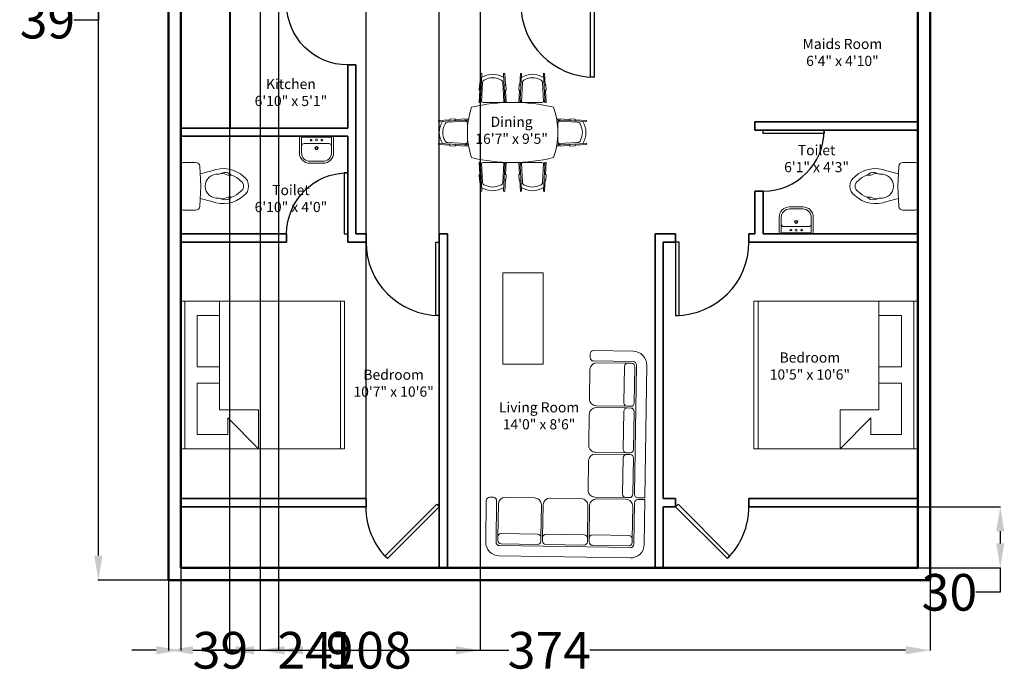
# Model space of a CAD drawing. Units: inches. Extents: x -230 to 384, y -962 to -183.
# Tile 1 of 6: x -175 to 309, y -962 to -640. Entities that reach past the tile are written whole.
import ezdxf

# ---------------------------------------------------------------- set-up
doc = ezdxf.new("R2010")
doc.units = ezdxf.units.IN
for name, color, linetype, lineweight in [('A-ANNO-DIMS', 2, 'Continuous', 18), ('A-AREA-IDEN', 7, 'Continuous', 18), ('A-DOOR', 3, 'Continuous', 25), ('A-FLOR-FIXT', 9, 'Continuous', 18), ('Furniture', 2, 'Continuous', 18), ('Inner Wall', 5, 'Continuous', 35), ('Kitchen', 4, 'Continuous', 25), ('Outer Wall', 1, 'Continuous', 50)]:
    doc.layers.add(name, color=color, linetype=linetype, lineweight=lineweight)
doc.styles.get("Standard").update_dxf_attribs({"font": 'arial.ttf'})
doc.dimstyles.get("Standard").update_dxf_attribs({"dimtxt": 18, "dimasz": 12, "dimexe": 0.18, "dimexo": 0.0625, "dimgap": 0.09, "dimtad": 0, "dimtih": 1, "dimtoh": 1, "dimdec": 0, "dimzin": 0, "dimdsep": 46, "dimlunit": 3, "dimtxsty": 'Standard', "dimcen": 0.09, "dimadec": 0, "dimazin": 0, "dimtfac": 1, "dimtdec": 0, "dimtofl": 0, "dimtmove": 0, "dimatfit": 3, "dimfxl": 1, "dimtolj": 1, "dimtzin": 0, "dimarcsym": 0})

# ---------------------------------------------------------------- blocks, each defined once
blk = doc.blocks.new('*U4')
for p, q in [((0, 0), (0, -4)), ((36, 0), (36, -4))]:
    blk.add_line(p, q)
blk.add_lwpolyline([(0, 0), (0, 36), (1.75, 36), (1.75, 0)], close=True)
blk.add_arc((0, 0), 36, 0, 90)
blk = doc.blocks.new('*U2')
for p, q in [((0, 0), (0, 4)), ((36, 0), (36, 4))]:
    blk.add_line(p, q)
blk.add_lwpolyline([(0, 0), (0, -36), (1.75, -36), (1.75, 0)], close=True)
blk.add_arc((0, 0), 36, 270, 0)
blk = doc.blocks.new('*U5')
for p, q in [((0, 0), (0, 4)), ((36, 0), (36, 4))]:
    blk.add_line(p, q)
blk.add_lwpolyline([(0, 0), (25.46, -25.46), (26.69, -24.22), (1.24, 1.24)], close=True)
blk.add_arc((0, 0), 36, 315, 0)
blk = doc.blocks.new('*U6')
for p, q in [((0, 0), (0, -4)), ((30, 0), (30, -4))]:
    blk.add_line(p, q)
blk.add_lwpolyline([(0, 0), (0, 30), (1.75, 30), (1.75, 0)], close=True)
blk.add_arc((0, 0), 30, 0, 90)
blk = doc.blocks.new('KING-00')
for p, q in [((-0.897, -0.947), (-0.897, 0.882)), ((0.602, 0.882), (0.602, -0.464)), ((1.034, -0.947), (1.034, 0.882)), ((0.602, 0.704), (0.881, 0.704)), ((0.881, 0.069), (0.881, 0.704)), ((0.602, 0.069), (0.881, 0.069)), ((0.881, -0.134), (0.602, -0.134)), ((0.881, -0.769), (0.881, -0.134)), ((0.119, -0.464), (0.119, -0.947)), ((0.602, -0.464), (0.119, -0.464)), ((0.119, -0.947), (0.5, -0.566)), ((0.5, -0.769), (0.5, -0.566)), ((0.5, -0.769), (0.881, -0.769))]:
    blk.add_line(p, q)
blk.add_lwpolyline([(-0.948, -0.947), (-0.948, 0.882), (1.084, 0.882), (1.084, -0.947)], close=True)
blk = doc.blocks.new('A$C1308471B')
at = {"ltscale": 20}
for p, q in [((0, 0.4607), (0, 0.0186)), ((0.0354, 0.4793), (0.1495, 0.4793)), ((0.2013, 0.2397), (0.1923, 0.4384)), ((0.1957, 0.3639), (0.3109, 0.3953)), ((0.5021, 0.3528), (0.4724, 0.3528)), ((0.4982, 0.3575), (0.4822, 0.3709)), ((0.2013, 0.2397), (0.1923, 0.0409)), ((0.1959, 0.1193), (0.3109, 0.0879)), ((0.5021, 0.1304), (0.4724, 0.1304)), ((0.4982, 0.1257), (0.4822, 0.1123)), ((0.0354, 0), (0.1495, 0))]:
    blk.add_line(p, q, dxfattribs=at)
for centre, radius, start, end in [((0.006, 0.4607), 0.006, 136.52689, 180), ((0.0354, 0.4328), 0.0465, 90, 136.52689), ((0.1495, 0.4365), 0.0429, 2.57554, 90), ((0.4248, 0.1104), 0.3068, 47.41345, 111.79241), ((0.3654, 0.2416), 0.1206, 83.35226, 180), ((0.3823, 0.3868), 0.0255, 263.35226, 298.57415), ((0.4494, 0.2636), 0.1148, 79.39683, 118.57415), ((0.405, 0.2159), 0.153, 63.50202, 90.45216), ((0.4658, 0.3513), 0.0255, 50, 79.39683), ((0.5146, 0.377), 0.0255, 230, 251.38812), ((0.5021, 0.3273), 0.0255, 70.3751, 90), ((0.4248, 0.1104), 0.2558, 46.61198, 70.3751), ((0.5654, 0.2416), 0.116, 0, 54.71147), ((0.3654, 0.2416), 0.1206, 180, 276.64774), ((0.5654, 0.2416), 0.065, 0, 57.29738), ((0.5654, 0.2416), 0.065, 302.70262, 0), ((0.5654, 0.2416), 0.116, 305.28853, 0), ((0.4248, 0.3728), 0.3068, 248.20759, 312.58655), ((0.3823, 0.0964), 0.0255, 61.42585, 96.64774), ((0.4494, 0.2196), 0.1148, 241.42585, 280.60317), ((0.405, 0.2673), 0.153, 269.54784, 296.49798), ((0.4658, 0.1319), 0.0255, 280.60317, 310), ((0.5146, 0.1062), 0.0255, 108.61188, 130), ((0.5021, 0.1559), 0.0255, 270, 289.6249), ((0.4248, 0.3728), 0.2558, 289.6249, 313.38802), ((0.006, 0.0186), 0.006, 180, 223.47311), ((0.0354, 0.0465), 0.0465, 223.47311, 270), ((0.1495, 0.0429), 0.0429, 270, 357.42446)]:
    blk.add_arc(centre, radius, start, end, dxfattribs=at)
blk = doc.blocks.new('A$C57EA129C')
for p, q in [((0, 0.443), (0, 0.178)), ((0.016, 0.459), (0.563, 0.459)), ((0.036, 0.432), (0.036, 0.29)), ((0.045, 0.441), (0.535, 0.441)), ((0.08, 0.334), (0.499, 0.334)), ((0.544, 0.432), (0.544, 0.29)), ((0.579, 0.443), (0.579, 0.178)), ((0.036, 0.29), (0.036, 0.178)), ((0.544, 0.29), (0.544, 0.178)), ((0.178, 0.036), (0.401, 0.036)), ((0.178, 0), (0.401, 0))]:
    blk.add_line(p, q)
for centre, radius in [((0.198, 0.392), 0.0143), ((0.29, 0.396), 0.0156), ((0.381, 0.392), 0.0143), ((0.29, 0.255), 0.0267), ((0.29, 0.255), 0.0178)]:
    blk.add_circle(centre, radius)
for centre, radius, start, end in [((0.016, 0.443), 0.016, 90, 180), ((0.045, 0.432), 0.00891, 90, 180), ((0.08, 0.29), 0.0445, 90, 180), ((0.499, 0.29), 0.0445, 0, 90), ((0.535, 0.432), 0.00891, 0, 90), ((0.563, 0.443), 0.016, 0, 90), ((0.178, 0.178), 0.178, 180, 270), ((0.178, 0.178), 0.143, 180, 270), ((0.401, 0.178), 0.178, 270, 0), ((0.401, 0.178), 0.143, 270, 0)]:
    blk.add_arc(centre, radius, start, end)
blk = doc.blocks.new('A$C2AFA021D')
for p, q in [((0.8, 2.3), (0.2, 2.3)), ((0.2, 2.15), (0.8, 2.15)), ((0.85, 2.2), (0.85, 2.25)), ((0, 2.1), (0, 0.2)), ((0.15, 0.2), (0.15, 2.1)), ((0.175, 1.55), (0.175, 2.075)), ((0.225, 2.125), (0.275, 2.125)), ((0.75, 2.125), (0.275, 2.125)), ((0.325, 2.075), (0.325, 1.55)), ((0.85, 1.6), (0.85, 2.025)), ((0.275, 1.5), (0.225, 1.5)), ((0.225, 1.475), (0.275, 1.475)), ((0.275, 1.5), (0.75, 1.5)), ((0.75, 1.475), (0.275, 1.475)), ((0.175, 0.875), (0.175, 1.425)), ((0.325, 1.425), (0.325, 0.875)), ((0.85, 0.925), (0.85, 1.375)), ((0.175, 0.225), (0.175, 0.75)), ((0.275, 0.825), (0.225, 0.825)), ((0.225, 0.8), (0.275, 0.8)), ((0.275, 0.825), (0.75, 0.825)), ((0.75, 0.8), (0.275, 0.8)), ((0.325, 0.75), (0.325, 0.225)), ((0.875, 0.275), (0.875, 0.725)), ((0.975, 0.825), (1.4, 0.825)), ((1.5, 0.725), (1.5, 0.275)), ((1.525, 0.275), (1.525, 0.725)), ((1.625, 0.825), (2.075, 0.825)), ((2.175, 0.725), (2.175, 0.275)), ((2.2, 0.275), (2.2, 0.725)), ((2.3, 0.825), (2.725, 0.825)), ((2.825, 0.725), (2.825, 0.275)), ((2.85, 0.2), (2.85, 0.775)), ((2.9, 0.825), (2.95, 0.825)), ((3, 0.775), (3, 0.2)), ((0.85, 0.275), (0.85, 0.7)), ((1.45, 0.325), (0.925, 0.325)), ((2.125, 0.325), (1.575, 0.325)), ((2.775, 0.325), (2.25, 0.325)), ((0.8, 0.15), (0.2, 0.15)), ((0.275, 0.175), (0.225, 0.175)), ((0.275, 0.175), (0.75, 0.175)), ((0.875, 0.275), (0.875, 0.225)), ((0.925, 0.175), (1.45, 0.175)), ((0.925, 0.15), (2.8, 0.15)), ((1.5, 0.225), (1.5, 0.275)), ((1.525, 0.275), (1.525, 0.225)), ((1.575, 0.175), (2.125, 0.175)), ((2.175, 0.225), (2.175, 0.275)), ((2.2, 0.275), (2.2, 0.225)), ((2.25, 0.175), (2.775, 0.175)), ((2.825, 0.225), (2.825, 0.275)), ((0.85, 0), (0.85, 0.1)), ((0.875, 0.1), (0.875, 0)), ((0.2, 0), (0.85, 0)), ((2.8, 0), (0.875, 0))]:
    blk.add_line(p, q)
for centre, radius, start, end in [((0.2, 2.1), 0.2, 90, 180), ((0.8, 2.25), 0.05, 0, 90), ((0.2, 2.1), 0.05, 90, 180), ((0.8, 2.2), 0.05, 270, 0), ((0.225, 2.075), 0.05, 90, 180), ((0.275, 2.075), 0.05, 0, 90), ((0.75, 2.025), 0.1, 0, 90), ((0.75, 1.6), 0.1, 270, 0), ((0.225, 1.55), 0.05, 180, 270), ((0.225, 1.425), 0.05, 90, 180), ((0.275, 1.55), 0.05, 270, 0), ((0.275, 1.425), 0.05, 0, 90), ((0.75, 1.375), 0.1, 360, 90), ((0.225, 0.875), 0.05, 180, 270), ((0.275, 0.875), 0.05, 270, 0), ((0.75, 0.925), 0.1, 270, 0), ((0.225, 0.75), 0.05, 90, 180), ((0.275, 0.75), 0.05, 0, 90), ((0.75, 0.7), 0.1, 0, 90), ((0.975, 0.725), 0.1, 90, 180), ((1.4, 0.725), 0.1, 0, 90), ((1.625, 0.725), 0.1, 90, 180), ((2.075, 0.725), 0.1, 0, 90), ((2.3, 0.725), 0.1, 90, 180), ((2.725, 0.725), 0.1, 0, 90), ((2.9, 0.775), 0.05, 90, 180), ((2.95, 0.775), 0.05, 0, 90), ((0.925, 0.275), 0.05, 90, 180), ((1.45, 0.275), 0.05, 360, 90), ((1.575, 0.275), 0.05, 90, 180), ((2.125, 0.275), 0.05, 360, 90), ((2.25, 0.275), 0.05, 90, 180), ((2.775, 0.275), 0.05, 360, 90), ((0.2, 0.2), 0.2, 180, 270), ((0.2, 0.2), 0.05, 180, 270), ((0.225, 0.225), 0.05, 180, 270), ((0.275, 0.225), 0.05, 270, 0), ((0.75, 0.275), 0.1, 270, 0), ((0.8, 0.1), 0.05, 0, 90), ((0.925, 0.225), 0.05, 180, 270), ((0.925, 0.1), 0.05, 90, 180), ((1.45, 0.225), 0.05, 270, 0), ((1.575, 0.225), 0.05, 180, 270), ((2.125, 0.225), 0.05, 270, 0), ((2.25, 0.225), 0.05, 180, 270), ((2.775, 0.225), 0.05, 270, 0), ((2.8, 0.2), 0.2, 270, 0), ((2.8, 0.2), 0.05, 270, 0)]:
    blk.add_arc(centre, radius, start, end)
blk = doc.blocks.new('A$C6BEF12A9')
for p, q in [((0.698, 1.955), (0.688, 1.768)), ((0.712, 1.841), (0.695, 1.529)), ((0.712, 1.841), (0.695, 1.529)), ((0.698, 1.955), (0.718, 1.954)), ((0.718, 1.954), (0.712, 1.841)), ((0.73, 1.806), (0.713, 1.488)), ((1.067, 1.806), (1.084, 1.488)), ((1.099, 1.955), (1.079, 1.954)), ((1.079, 1.954), (1.085, 1.841)), ((1.085, 1.841), (1.102, 1.529)), ((1.099, 1.955), (1.109, 1.768)), ((1.358, 1.955), (1.349, 1.768)), ((1.372, 1.841), (1.356, 1.529)), ((1.372, 1.841), (1.356, 1.529)), ((1.358, 1.955), (1.378, 1.954)), ((1.378, 1.954), (1.372, 1.841)), ((1.391, 1.806), (1.374, 1.488)), ((1.728, 1.806), (1.744, 1.488)), ((1.76, 1.955), (1.74, 1.954)), ((1.74, 1.954), (1.746, 1.841)), ((1.746, 1.841), (1.762, 1.529)), ((1.76, 1.955), (1.77, 1.768)), ((0.678, 1.768), (0.673, 1.678)), ((0.683, 1.678), (0.673, 1.477)), ((0.703, 1.678), (0.673, 1.678)), ((0.708, 1.768), (0.678, 1.768)), ((1.089, 1.768), (1.119, 1.768)), ((1.094, 1.678), (1.124, 1.678)), ((1.114, 1.678), (1.124, 1.477)), ((1.119, 1.768), (1.124, 1.678)), ((1.344, 1.678), (1.333, 1.477)), ((1.339, 1.768), (1.334, 1.678)), ((1.364, 1.678), (1.334, 1.678)), ((1.369, 1.768), (1.339, 1.768)), ((1.75, 1.768), (1.78, 1.768)), ((1.754, 1.678), (1.784, 1.678)), ((1.774, 1.678), (1.785, 1.477)), ((1.78, 1.768), (1.784, 1.678)), ((0.673, 1.477), (0.693, 1.476)), ((0.693, 1.476), (0.695, 1.526)), ((0.745, 1.476), (1.052, 1.476)), ((1.104, 1.476), (1.102, 1.526)), ((1.124, 1.477), (1.104, 1.476)), ((1.333, 1.477), (1.353, 1.476)), ((1.353, 1.476), (1.356, 1.526)), ((1.406, 1.476), (1.712, 1.476)), ((1.765, 1.476), (1.762, 1.526)), ((1.785, 1.477), (1.765, 1.476)), ((0, 1.178), (0.187, 1.188)), ((0, 1.178), (0.001, 1.158)), ((0.001, 1.158), (0.114, 1.164)), ((0.114, 1.164), (0.426, 1.181)), ((0.149, 1.146), (0.467, 1.163)), ((0.187, 1.198), (0.277, 1.203)), ((0.187, 1.168), (0.187, 1.198)), ((0.277, 1.193), (0.477, 1.203)), ((0.277, 1.173), (0.277, 1.203)), ((0.479, 1.183), (0.429, 1.181)), ((0.477, 1.203), (0.479, 1.183)), ((1.98, 1.203), (1.979, 1.183)), ((1.979, 1.183), (2.029, 1.181)), ((2.18, 1.193), (1.98, 1.203)), ((2.309, 1.146), (1.99, 1.163)), ((2.343, 1.164), (2.031, 1.181)), ((2.18, 1.173), (2.18, 1.203)), ((2.27, 1.198), (2.18, 1.203)), ((2.27, 1.168), (2.27, 1.198)), ((2.458, 1.178), (2.27, 1.188)), ((2.457, 1.158), (2.343, 1.164)), ((2.458, 1.178), (2.457, 1.158)), ((0.479, 0.824), (0.479, 1.131)), ((1.979, 0.824), (1.979, 1.131)), ((0, 0.777), (0.001, 0.797)), ((0, 0.777), (0.187, 0.767)), ((0.001, 0.797), (0.114, 0.791)), ((0.114, 0.791), (0.426, 0.774)), ((0.114, 0.791), (0.426, 0.774)), ((0.149, 0.809), (0.467, 0.792)), ((0.187, 0.787), (0.187, 0.757)), ((0.187, 0.757), (0.277, 0.752)), ((0.277, 0.782), (0.277, 0.752)), ((0.277, 0.762), (0.477, 0.752)), ((0.479, 0.772), (0.429, 0.774)), ((0.477, 0.752), (0.479, 0.772)), ((1.979, 0.772), (2.029, 0.774)), ((1.98, 0.752), (1.979, 0.772)), ((2.18, 0.762), (1.98, 0.752)), ((2.309, 0.809), (1.99, 0.792)), ((2.343, 0.791), (2.031, 0.774)), ((2.343, 0.791), (2.031, 0.774)), ((2.18, 0.782), (2.18, 0.752)), ((2.27, 0.757), (2.18, 0.752)), ((2.27, 0.787), (2.27, 0.757)), ((2.458, 0.777), (2.27, 0.767)), ((2.457, 0.797), (2.343, 0.791)), ((2.458, 0.777), (2.457, 0.797)), ((0.673, 0.477), (0.693, 0.479)), ((0.683, 0.277), (0.673, 0.477)), ((0.693, 0.479), (0.695, 0.429)), ((0.712, 0.114), (0.695, 0.426)), ((0.712, 0.114), (0.695, 0.426)), ((0.73, 0.149), (0.713, 0.467)), ((0.745, 0.479), (1.052, 0.479)), ((1.067, 0.149), (1.084, 0.467)), ((1.085, 0.114), (1.102, 0.426)), ((1.104, 0.479), (1.102, 0.429)), ((1.124, 0.477), (1.104, 0.479)), ((1.114, 0.277), (1.124, 0.477)), ((1.333, 0.477), (1.353, 0.479)), ((1.344, 0.277), (1.333, 0.477)), ((1.353, 0.479), (1.356, 0.429)), ((1.372, 0.114), (1.356, 0.426)), ((1.372, 0.114), (1.356, 0.426)), ((1.391, 0.149), (1.374, 0.467)), ((1.406, 0.479), (1.712, 0.479)), ((1.728, 0.149), (1.744, 0.467)), ((1.746, 0.114), (1.762, 0.426)), ((1.765, 0.479), (1.762, 0.429)), ((1.785, 0.477), (1.765, 0.479)), ((1.774, 0.277), (1.785, 0.477)), ((0.678, 0.187), (0.673, 0.277)), ((0.703, 0.277), (0.673, 0.277)), ((0.708, 0.187), (0.678, 0.187)), ((0.698, 0), (0.688, 0.187)), ((1.089, 0.187), (1.119, 0.187)), ((1.094, 0.277), (1.124, 0.277)), ((1.099, 0), (1.109, 0.187)), ((1.119, 0.187), (1.124, 0.277)), ((1.364, 0.277), (1.334, 0.277)), ((1.339, 0.187), (1.334, 0.277)), ((1.369, 0.187), (1.339, 0.187)), ((1.358, 0), (1.349, 0.187)), ((1.75, 0.187), (1.78, 0.187)), ((1.754, 0.277), (1.784, 0.277)), ((1.76, 0), (1.77, 0.187)), ((1.78, 0.187), (1.784, 0.277)), ((0.698, 0), (0.718, 0.001)), ((0.718, 0.001), (0.712, 0.114)), ((1.079, 0.001), (1.085, 0.114)), ((1.099, 0), (1.079, 0.001)), ((1.358, 0), (1.378, 0.001)), ((1.378, 0.001), (1.372, 0.114)), ((1.74, 0.001), (1.746, 0.114)), ((1.76, 0), (1.74, 0.001))]:
    blk.add_line(p, q)
for centre, radius, start, end in [((0.898, 1.603), 0.341, 57.3412, 122.6588), ((0.78, 1.804), 0.05, 103.7138, 177), ((0.898, 1.603), 0.281, 62.3651, 117.6349), ((1.017, 1.804), 0.05, 3, 76.2862), ((1.559, 1.603), 0.341, 57.3412, 122.6588), ((1.441, 1.804), 0.05, 103.7138, 177), ((1.559, 1.603), 0.281, 62.3651, 117.6349), ((1.678, 1.804), 0.05, 3, 76.2862), ((1.229, -1.385), 2.862, 76.2365, 103.7635), ((0.745, 1.526), 0.05, 177, 270), ((1.052, 1.526), 0.05, 270, 3), ((1.406, 1.526), 0.05, 177, 270), ((1.712, 1.526), 0.05, 270, 3), ((1.779, 0.977), 1.3, 161.253, 198.747), ((0.679, 0.977), 1.3, 341.253, 18.747), ((0.352, 0.977), 0.341, 147.3412, 212.6588), ((0.151, 1.096), 0.05, 93, 166.2862), ((0.429, 1.131), 0.05, 0, 93), ((2.029, 1.131), 0.05, 87, 180), ((2.306, 1.096), 0.05, 13.7138, 87), ((2.106, 0.977), 0.341, 327.3412, 32.6588), ((0.352, 0.977), 0.281, 152.3651, 207.6349), ((2.106, 0.977), 0.281, 332.3651, 27.6349), ((0.151, 0.859), 0.05, 193.7138, 267), ((0.429, 0.824), 0.05, 267, 0), ((2.029, 0.824), 0.05, 180, 273), ((2.306, 0.859), 0.05, 273, 346.2862), ((1.229, 3.34), 2.862, 256.2365, 283.7635), ((0.745, 0.429), 0.05, 90, 183), ((1.052, 0.429), 0.05, 357, 90), ((1.406, 0.429), 0.05, 90, 183), ((1.712, 0.429), 0.05, 357, 90), ((0.898, 0.352), 0.341, 237.3412, 302.6588), ((0.78, 0.151), 0.05, 183, 256.2862), ((0.898, 0.352), 0.281, 242.3651, 297.6349), ((1.017, 0.151), 0.05, 283.7138, 357), ((1.559, 0.352), 0.341, 237.3412, 302.6588), ((1.441, 0.151), 0.05, 183, 256.2862), ((1.559, 0.352), 0.281, 242.3651, 297.6349), ((1.678, 0.151), 0.05, 283.7138, 357)]:
    blk.add_arc(centre, radius, start, end)
blk = doc.blocks.new('TABLE-COFFEE-RECT')
blk.add_lwpolyline([(0, 44.94), (19.86, 44.94), (19.86, 0), (0, 0)], close=True)
blk = doc.blocks.new('*D32')
at = {"layer": 'A-ANNO-DIMS', "color": 0, "lineweight": -2, "transparency": 16777216}
for p, q in [((-101.6, -915.32), (-101.6, -949.88)), ((272.4, -915.32), (272.4, -949.88)), ((-89.6, -949.7), (65.47, -949.7)), ((260.4, -949.7), (105.33, -949.7))]:
    blk.add_line(p, q, dxfattribs=at)
at = {"layer": 'A-ANNO-DIMS', "color": 0, "transparency": 16777216}
for points in [[(-89.6, -947.7), (-89.6, -951.7), (-101.6, -949.7)], [(260.4, -947.7), (260.4, -951.7), (272.4, -949.7)]]:
    blk.add_solid(points, dxfattribs=at)
at = {"layer": 'Defpoints', "color": 0, "transparency": 16777216}
for p in [(-101.6, -915.25), (272.4, -915.25), (272.4, -949.7)]:
    blk.add_point(p, dxfattribs=at)
at = {"layer": 'A-ANNO-DIMS', "color": 0, "transparency": 16777216, "insert": (85.4, -949.7), "char_height": 18, "attachment_point": 5}
blk.add_mtext('\\A1;374', dxfattribs=at)
blk = doc.blocks.new('*D33')
at = {"layer": 'A-ANNO-DIMS', "color": 0, "lineweight": -2, "transparency": 16777216}
for p, q in [((-101.66, -229.25), (-136.23, -229.25)), ((-136.05, -241.25), (-136.05, -562.97)), ((-136.05, -903.25), (-136.05, -581.53)), ((-101.66, -915.25), (-136.23, -915.25))]:
    blk.add_line(p, q, dxfattribs=at)
at = {"layer": 'A-ANNO-DIMS', "color": 0, "transparency": 16777216}
for points in [[(-138.05, -241.25), (-134.05, -241.25), (-136.05, -229.25)], [(-138.05, -903.25), (-134.05, -903.25), (-136.05, -915.25)]]:
    blk.add_solid(points, dxfattribs=at)
at = {"layer": 'Defpoints', "color": 0, "transparency": 16777216}
for p in [(-101.6, -229.25), (-136.05, -915.25), (-101.6, -915.25)]:
    blk.add_point(p, dxfattribs=at)
at = {"layer": 'A-ANNO-DIMS', "color": 0, "transparency": 16777216, "insert": (-136.05, -572.25), "char_height": 18, "attachment_point": 5}
blk.add_mtext('\\A1;686', dxfattribs=at)
blk = doc.blocks.new('*D38')
at = {"layer": 'A-ANNO-DIMS', "color": 0, "lineweight": -2, "transparency": 16777216}
for p, q in [((-56.6, -628.32), (-56.6, -949.88)), ((51.4, -628.32), (51.4, -949.88)), ((-44.6, -949.7), (-21.75, -949.7)), ((39.4, -949.7), (16.54, -949.7))]:
    blk.add_line(p, q, dxfattribs=at)
at = {"layer": 'A-ANNO-DIMS', "color": 0, "transparency": 16777216}
for points in [[(-44.6, -947.7), (-44.6, -951.7), (-56.6, -949.7)], [(39.4, -947.7), (39.4, -951.7), (51.4, -949.7)]]:
    blk.add_solid(points, dxfattribs=at)
at = {"layer": 'Defpoints', "color": 0, "transparency": 16777216}
for p in [(-56.6, -628.25), (51.4, -628.25), (51.4, -949.7)]:
    blk.add_point(p, dxfattribs=at)
at = {"layer": 'A-ANNO-DIMS', "color": 0, "transparency": 16777216, "insert": (-2.6, -949.7), "char_height": 18, "attachment_point": 5}
blk.add_mtext('\\A1;108', dxfattribs=at)
blk = doc.blocks.new('*D39')
at = {"layer": 'A-ANNO-DIMS', "color": 0, "lineweight": -2, "transparency": 16777216}
for p, q in [((-56.66, -589.25), (-136.23, -589.25)), ((-136.05, -601.25), (-136.05, -616.25)), ((-56.66, -628.25), (-136.23, -628.25)), ((-136.05, -628.25), (-136.05, -640.25)), ((-136.05, -640.25), (-148.05, -640.25))]:
    blk.add_line(p, q, dxfattribs=at)
at = {"layer": 'A-ANNO-DIMS', "color": 0, "transparency": 16777216}
for points in [[(-138.05, -601.25), (-134.05, -601.25), (-136.05, -589.25)], [(-138.05, -616.25), (-134.05, -616.25), (-136.05, -628.25)]]:
    blk.add_solid(points, dxfattribs=at)
at = {"layer": 'Defpoints', "color": 0, "transparency": 16777216}
for p in [(-56.6, -589.25), (-136.05, -628.25), (-56.6, -628.25)]:
    blk.add_point(p, dxfattribs=at)
at = {"layer": 'A-ANNO-DIMS', "color": 0, "transparency": 16777216, "insert": (-161.05, -640.25), "char_height": 18, "attachment_point": 5}
blk.add_mtext('\\A1;39', dxfattribs=at)
blk = doc.blocks.new('*D40')
at = {"layer": 'A-ANNO-DIMS', "color": 0, "lineweight": -2, "transparency": 16777216}
for p, q in [((266.46, -879.25), (307.03, -879.25)), ((306.85, -891.25), (306.85, -897.25)), ((266.46, -909.25), (307.03, -909.25)), ((306.85, -909.25), (306.85, -921.25)), ((306.85, -921.25), (294.85, -921.25))]:
    blk.add_line(p, q, dxfattribs=at)
at = {"layer": 'A-ANNO-DIMS', "color": 0, "transparency": 16777216}
for points in [[(304.85, -891.25), (308.85, -891.25), (306.85, -879.25)], [(304.85, -897.25), (308.85, -897.25), (306.85, -909.25)]]:
    blk.add_solid(points, dxfattribs=at)
at = {"layer": 'Defpoints', "color": 0, "transparency": 16777216}
for p in [(266.4, -879.25), (266.4, -909.25), (306.85, -909.25)]:
    blk.add_point(p, dxfattribs=at)
at = {"layer": 'A-ANNO-DIMS', "color": 0, "transparency": 16777216, "insert": (281.9, -921.25), "char_height": 18, "attachment_point": 5}
blk.add_mtext('\\A1;30', dxfattribs=at)
blk = doc.blocks.new('*D41')
at = {"layer": 'A-ANNO-DIMS', "color": 0, "lineweight": -2, "transparency": 16777216}
for p, q in [((-95.6, -454.32), (-95.6, -949.88)), ((-71.6, -454.32), (-71.6, -949.88)), ((-107.6, -949.7), (-119.6, -949.7)), ((-59.6, -949.7), (-47.6, -949.7))]:
    blk.add_line(p, q, dxfattribs=at)
at = {"layer": 'A-ANNO-DIMS', "color": 0, "transparency": 16777216}
for points in [[(-107.6, -947.7), (-107.6, -951.7), (-95.6, -949.7)], [(-59.6, -947.7), (-59.6, -951.7), (-71.6, -949.7)]]:
    blk.add_solid(points, dxfattribs=at)
at = {"layer": 'Defpoints', "color": 0, "transparency": 16777216}
for p in [(-95.6, -454.25), (-71.6, -454.25), (-71.6, -949.7)]:
    blk.add_point(p, dxfattribs=at)
at = {"layer": 'A-ANNO-DIMS', "color": 0, "transparency": 16777216, "insert": (-34.5, -949.7), "char_height": 18, "attachment_point": 5}
blk.add_mtext('\\A1;24', dxfattribs=at)
blk = doc.blocks.new('*D46')
at = {"layer": 'A-ANNO-DIMS', "color": 0, "lineweight": -2, "transparency": 16777216}
for p, q in [((-56.6, -577.32), (-56.6, -949.88)), ((-47.6, -577.32), (-47.6, -949.88)), ((-68.6, -949.7), (-80.6, -949.7)), ((-35.6, -949.7), (-23.6, -949.7))]:
    blk.add_line(p, q, dxfattribs=at)
at = {"layer": 'A-ANNO-DIMS', "color": 0, "transparency": 16777216}
for points in [[(-68.6, -947.7), (-68.6, -951.7), (-56.6, -949.7)], [(-35.6, -947.7), (-35.6, -951.7), (-47.6, -949.7)]]:
    blk.add_solid(points, dxfattribs=at)
at = {"layer": 'Defpoints', "color": 0, "transparency": 16777216}
for p in [(-56.6, -577.25), (-47.6, -577.25), (-47.6, -949.7)]:
    blk.add_point(p, dxfattribs=at)
at = {"layer": 'A-ANNO-DIMS', "color": 0, "transparency": 16777216, "insert": (-17.59, -949.7), "char_height": 18, "attachment_point": 5}
blk.add_mtext('\\A1;9', dxfattribs=at)
blk = doc.blocks.new('*D47')
at = {"layer": 'A-ANNO-DIMS', "color": 0, "lineweight": -2, "transparency": 16777216}
for p, q in [((-95.60199, -628.31695), (-95.60199, -949.88445)), ((-56.60199, -628.31695), (-56.60199, -949.88445)), ((-107.60199, -949.70445), (-119.60199, -949.70445)), ((-44.60199, -949.70445), (-32.60199, -949.70445))]:
    blk.add_line(p, q, dxfattribs=at)
at = {"layer": 'A-ANNO-DIMS', "color": 0, "transparency": 16777216}
for points in [[(-107.60199, -947.70445), (-107.60199, -951.70445), (-95.60199, -949.70445)], [(-44.60199, -947.70445), (-44.60199, -951.70445), (-56.60199, -949.70445)]]:
    blk.add_solid(points, dxfattribs=at)
at = {"layer": 'Defpoints', "color": 0, "transparency": 16777216}
for p in [(-95.60199, -628.25445), (-56.60199, -628.25445), (-56.60199, -949.70445)]:
    blk.add_point(p, dxfattribs=at)
at = {"layer": 'A-ANNO-DIMS', "color": 0, "transparency": 16777216, "insert": (-76.10199, -949.70445), "char_height": 18, "attachment_point": 5}
blk.add_mtext('\\A1;39', dxfattribs=at)
blk = doc.blocks.new('*D51')
at = {"layer": 'A-ANNO-DIMS', "color": 0, "lineweight": -2, "transparency": 16777216}
for p, q in [((-16.60199, -194.80445), (-28.60199, -194.80445)), ((-4.60199, -875.19195), (-4.60199, -194.62445)), ((31.39801, -875.19195), (31.39801, -194.62445)), ((43.39801, -194.80445), (55.39801, -194.80445))]:
    blk.add_line(p, q, dxfattribs=at)
at = {"layer": 'A-ANNO-DIMS', "color": 0, "transparency": 16777216}
for points in [[(-16.60199, -192.80445), (-16.60199, -196.80445), (-4.60199, -194.80445)], [(43.39801, -192.80445), (43.39801, -196.80445), (31.39801, -194.80445)]]:
    blk.add_solid(points, dxfattribs=at)
at = {"layer": 'Defpoints', "color": 0, "transparency": 16777216}
for p in [(31.39801, -194.80445), (-4.60199, -875.25445), (31.39801, -875.25445)]:
    blk.add_point(p, dxfattribs=at)
at = {"layer": 'A-ANNO-DIMS', "color": 0, "transparency": 16777216, "insert": (13.39801, -194.80445), "char_height": 18, "attachment_point": 5}
blk.add_mtext('\\A1;36', dxfattribs=at)

msp = doc.modelspace()

# ---------------------------------------------------------------- linework, layer by layer
at = {"layer": 'Inner Wall'}
for p, q in [((-13.6, -693.25), (-13.6, -662.25)), ((-13.6, -662.25), (-9.6, -662.25)), ((-9.6, -745.25), (-9.6, -662.25)), ((186.4, -690.25), (266.4, -690.25)), ((186.4, -690.25), (186.4, -694.25)), ((-13.6, -693.25), (-95.6, -693.25)), ((186.4, -694.25), (266.4, -694.25)), ((-13.6, -697.25), (-95.6, -697.25)), ((-13.6, -749.25), (-13.6, -697.25)), ((186.4, -724.25), (190.4, -724.25)), ((186.4, -724.25), (186.4, -745.25)), ((190.4, -724.25), (190.4, -745.25)), ((-43.6, -745.25), (-95.6, -745.25)), ((-43.6, -749.25), (-95.6, -749.25)), ((-43.6, -749.25), (-43.6, -745.25)), ((-4.6, -749.25), (-13.6, -749.25)), ((-4.6, -745.25), (-9.6, -745.25)), ((-4.6, -749.25), (-4.6, -745.25)), ((31.4, -909.25), (31.4, -745.25)), ((35.4, -745.25), (31.4, -745.25)), ((35.4, -909.25), (35.4, -745.25)), ((137.4, -745.25), (147.4, -745.25)), ((137.4, -745.25), (137.4, -909.25)), ((141.4, -749.25), (147.4, -749.25)), ((141.4, -749.25), (141.4, -875.25)), ((147.4, -745.25), (147.4, -749.25)), ((183.4, -745.25), (183.4, -749.25)), ((183.4, -745.25), (186.4, -745.25)), ((183.4, -749.25), (266.4, -749.25)), ((190.4, -745.25), (266.4, -745.25)), ((-4.6, -875.25), (-95.6, -875.25)), ((-4.6, -879.25), (-95.6, -879.25)), ((-4.6, -875.25), (-4.6, -879.25)), ((141.4, -875.25), (147.4, -875.25)), ((141.4, -879.25), (147.4, -879.25)), ((141.4, -879.25), (141.4, -909.25)), ((147.4, -879.25), (147.4, -875.25)), ((183.4, -879.25), (183.4, -875.25)), ((183.4, -875.25), (266.4, -875.25)), ((183.4, -879.25), (266.4, -879.25))]:
    msp.add_line(p, q, dxfattribs=at)
at = {"layer": 'Kitchen'}
msp.add_lwpolyline([(-95.6, -632.25), (-71.3, -632.25), (-71.3, -693.25), (-95.6, -693.25)], close=True, dxfattribs=at)
at = {"layer": 'Outer Wall'}
for p, q in [((-95.6, -909.25), (-95.6, -235.25)), ((266.4, -235.25), (266.4, -909.25)), ((266.4, -909.25), (-95.6, -909.25))]:
    msp.add_line(p, q, dxfattribs=at)
msp.add_lwpolyline([(272.4, -915.25), (-101.6, -915.25), (-101.6, -229.25), (272.4, -229.25)], close=True, dxfattribs=at)

# ---------------------------------------------------------------- block references
at = {"layer": 'A-DOOR'}
for name, p, rotation in [('*U4', (107.4, -632.25), 180), ('*U6', (190.4, -694.25), 270), ('*U4', (31.4, -749.25), 180)]:
    msp.add_blockref(name, p, dxfattribs=dict(at, rotation=rotation))
at = {"layer": 'A-DOOR', "xscale": -1, "rotation": 90}
msp.add_blockref('*U6', (-13.6, -632.25), dxfattribs=at)
at = {"layer": 'A-DOOR', "xscale": -1}
for name, p in [('*U6', (-13.6, -745.25)), ('*U5', (31.4, -879.25))]:
    msp.add_blockref(name, p, dxfattribs=at)
at = {"layer": 'A-DOOR'}
for name, p in [('*U2', (147.4, -749.25)), ('*U5', (147.4, -879.25))]:
    msp.add_blockref(name, p, dxfattribs=at)
at = {"layer": 'A-FLOR-FIXT'}
for name, p, xscale, yscale, zscale in [('A$C57EA129C', (-20.52, -710.55), -28.98333223671166, 28.98333223671166, 28.98333223671166), ('A$C1308471B', (-95.6, -733.61), 48.95497407897215, 48.95497407897215, 48.95497407897215), ('A$C1308471B', (266.4, -733.61), -48.95497407897215, 48.95497407897215, 48.95497407897215)]:
    msp.add_blockref(name, p, dxfattribs=dict(at, xscale=xscale, yscale=yscale, zscale=zscale))
at = {"layer": 'A-FLOR-FIXT', "xscale": 28.98333223671166, "yscale": 28.98333223671166, "zscale": 28.98333223671166, "rotation": 180}
msp.add_blockref('A$C57EA129C', (215.06, -731.96), dxfattribs=at)
at = {"layer": 'Furniture'}
for name, p, xscale, yscale, zscale in [('A$C6BEF12A9', (31.01, -724.34), 29.59247402267948, 29.59247402267948, 29.59247402267948), ('KING-00', (-52.65, -813.22), -39.60249106241186, 39.60249106241186, 39.60249106241186), ('KING-00', (223.45, -813.22), 39.60249106241186, 39.60249106241186, 39.60249106241186)]:
    msp.add_blockref(name, p, dxfattribs=dict(at, xscale=xscale, yscale=yscale, zscale=zscale))
msp.add_blockref('TABLE-COFFEE-RECT', (62.58, -809.22), dxfattribs=at)
at = {"layer": 'Furniture', "xscale": 33.84012530478223, "yscale": 33.84012530478223, "zscale": 33.84012530478223, "rotation": 89.14549705207068}
msp.add_blockref('A$C2AFA021D', (131.9, -904.46), dxfattribs=at)

# ---------------------------------------------------------------- texts
at = {"layer": 'A-AREA-IDEN', "char_height": 5, "attachment_point": 3}
for s, insert in [('\\pxqc;{\\fTimes New Roman|b0|i0|c0|p18;Maids Room\\P6\'4" x 4\'10"}', (253.9, -649.44)), ('\\pxqc;{\\fTimes New Roman|b0|i0|c0|p18;Kitchen\\P6\'10" x 5\'1"}', (-16.93, -669.11)), ('\\pxqc;{\\fTimes New Roman|b0|i0|c0|p18;Dining\\P16\'7" x 9\'5"}', (91.45, -687.68)), ('\\pxqc;{\\fTimes New Roman|b0|i0|c0|p18;Toilet\\P6\'1" x 4\'3"}', (241.21, -701.6)), ('\\pxqc;{\\fTimes New Roman|b0|i0|c0|p18;Toilet\\P6\'10" x 4\'0"}', (-16.93, -721.2)), ('\\pxqc;{\\fTimes New Roman|b0|i0|c0|p18;Bedroom\\P10\'5" x 10\'6"}', (237.92, -803.45)), ('\\pxqc;{\\fTimes New Roman|b0|i0|c0|p18;Bedroom\\P10\'7" x 10\'6"}', (33.51, -811.87)), ('\\pxqc;{\\fTimes New Roman|b0|i0|c0|p18;Living Room\\P14\'0" x 8\'6"}', (104.92, -827.91))]:
    msp.add_mtext_dynamic_manual_height_columns(s, width=49.1019, gutter_width=12.5, heights=[0], dxfattribs=dict(at, insert=insert))

# ---------------------------------------------------------------- dimensions: what is measured, and where the dimension line sits
at = {"layer": 'A-ANNO-DIMS'}
for base, p1, p2, picture, middle in [((31.4, -194.8), (-4.6, -875.25), (31.4, -875.25), '*D51', (13.4, -194.8)), ((-71.6, -949.7), (-95.6, -454.25), (-71.6, -454.25), '*D41', (-34.5, -949.7)), ((-47.6, -949.7), (-56.6, -577.25), (-47.6, -577.25), '*D46', (-17.59, -949.7)), ((-56.6, -949.7), (-95.6, -628.25), (-56.6, -628.25), '*D47', (-76.1, -949.7)), ((51.4, -949.7), (-56.6, -628.25), (51.4, -628.25), '*D38', (-2.6, -949.7)), ((272.4, -949.7), (-101.6, -915.25), (272.4, -915.25), '*D32', (85.4, -949.7))]:
    dim = msp.add_linear_dim(base=base, p1=p1, p2=p2, dimstyle='Standard', override={"dimdec": 0, "dimlfac": 1, "dimrnd": 0, "dimzin": 0, "dimdsep": 46, "dimlunit": 2}, dxfattribs=at)
    dim.commit()
    dim.dimension.update_dxf_attribs({"geometry": picture, "text_midpoint": middle})
for base, p1, p2, picture, middle in [((-136.05, -915.25), (-101.6, -229.25), (-101.6, -915.25), '*D33', (-136.05, -572.25)), ((-136.05, -628.25), (-56.6, -589.25), (-56.6, -628.25), '*D39', (-161.05, -640.25)), ((306.85, -909.25), (266.4, -879.25), (266.4, -909.25), '*D40', (281.9, -921.25))]:
    dim = msp.add_linear_dim(base=base, p1=p1, p2=p2, angle=90, dimstyle='Standard', override={"dimdec": 0, "dimlfac": 1, "dimrnd": 0, "dimzin": 0, "dimdsep": 46, "dimlunit": 2}, dxfattribs=at)
    dim.commit()
    dim.dimension.update_dxf_attribs({"geometry": picture, "text_midpoint": middle})

doc.saveas('drawing.dxf')
